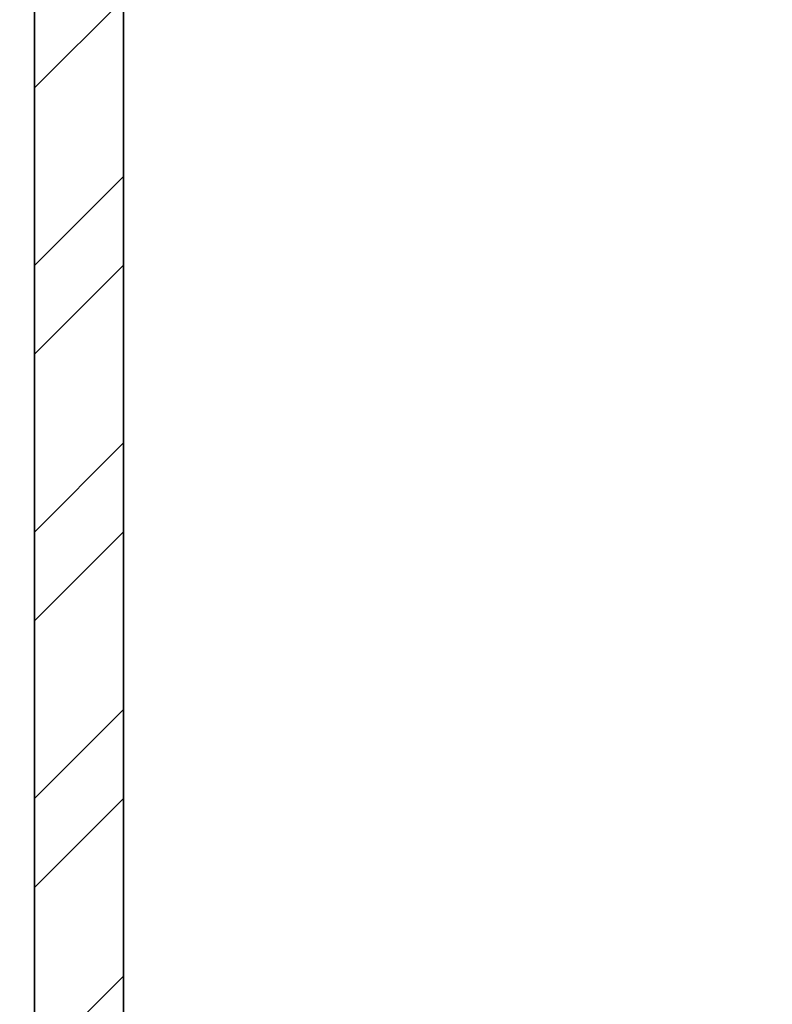
# Model space of a CAD drawing. Units: inches. Extents: x 1885 to 2748, y 783 to 2421.
# Tile 107 of 117: x 2486 to 2524, y 1977 to 2027. Entities that reach past the tile are written whole.
import ezdxf

# ---------------------------------------------------------------- set-up
doc = ezdxf.new("R2010")
doc.units = ezdxf.units.IN
doc.layers.add('A-WALL', color=7, linetype='Continuous', lineweight=35)
doc.layers.add('A-WALL-PATT', color=85, linetype='Continuous', lineweight=13, true_color=0x58ba48)

msp = doc.modelspace()

# ---------------------------------------------------------------- hatches: boundary and pattern name
at = {"layer": 'A-WALL-PATT'}
h = msp.add_hatch(dxfattribs=at)
h.set_pattern_fill('ANSI32', color=256)
h.paths.add_polyline_path([(2007.772, 2318.006), (1980.774, 2318.006), (1980.774, 2281.215), (1985.274, 2281.215), (1985.274, 2313.506), (2007.772, 2313.506), (2007.772, 2315.756)])
h.paths.add_polyline_path([(2094.324, 2318.006), (2067.772, 2318.006), (2067.772, 2313.506), (2094.324, 2313.506), (2094.324, 2315.756)])
h.paths.add_polyline_path([(2131.367, 2315.756), (2131.367, 2318.006), (2131.189, 2318.006), (2112.609, 2318.006), (2112.609, 2313.506), (2117.274, 2313.506), (2117.274, 2255.201), (2121.774, 2255.201), (2121.774, 2313.506), (2131.367, 2313.506)])
h.paths.add_polyline_path([(2190.512, 2318.006), (2155.367, 2318.006), (2155.367, 2313.506), (2169.774, 2313.506), (2169.774, 2229.506), (2121.774, 2229.506), (2121.774, 2233.451), (2119.524, 2233.451), (2117.274, 2233.451), (2117.274, 2201.101), (2121.774, 2201.101), (2121.774, 2225.006), (2169.774, 2225.006), (2169.774, 2165.006), (2306.274, 2165.006), (2306.274, 2066.006), (2310.774, 2066.006), (2344.274, 2066.006), (2486.274, 2066.006), (2486.274, 1886.006), (2483.02, 1886.006), (2483.02, 1881.506), (2486.274, 1881.506), (2486.274, 1880.678), (2490.774, 1880.678), (2490.774, 2070.506), (2344.274, 2070.506), (2310.774, 2070.506), (2310.774, 2165.006), (2310.774, 2173.636), (2308.524, 2173.636), (2306.274, 2173.636), (2306.274, 2169.506), (2174.274, 2169.506), (2174.274, 2313.506), (2190.512, 2313.506), (2190.512, 2315.756)])
h.paths.add_polyline_path([(1985.274, 2221.215), (1980.774, 2221.215), (1980.774, 2165.006), (1992.774, 2165.006), (1992.774, 2141.927), (1997.274, 2141.927), (1997.274, 2165.006), (2117.274, 2165.006), (2117.274, 2163.126), (2121.774, 2163.126), (2121.774, 2172.734), (2119.524, 2172.734), (2117.274, 2172.734), (2117.274, 2169.506), (1985.274, 2169.506)])
h.paths.add_polyline_path([(1997.274, 2105.927), (1992.774, 2105.927), (1992.774, 2070.506), (2016.774, 2070.506), (2016.774, 2059.123), (2019.024, 2059.123), (2021.274, 2059.123), (2021.274, 2070.506), (2117.274, 2070.506), (2117.274, 2022.506), (2114.423, 2022.506), (2114.423, 2018.006), (2123.627, 2018.006), (2123.627, 2020.256), (2123.627, 2022.506), (2121.774, 2022.506), (2121.774, 2142.587), (2119.524, 2142.587), (2117.274, 2142.587), (2117.274, 2075.006), (1997.274, 2075.006)])
h.paths.add_polyline_path([(2092.029, 2020.256), (2092.029, 2022.506), (2021.274, 2022.506), (2021.274, 2035.123), (2016.774, 2035.123), (2016.774, 2018.006), (2016.774, 1978.784), (2021.274, 1978.784), (2021.274, 2018.006), (2092.029, 2018.006)])
h.paths.add_polyline_path([(2260.938, 2022.506), (2153.105, 2022.506), (2153.105, 2020.256), (2153.105, 2018.006), (2155.274, 2018.006), (2155.274, 1886.006), (2107.629, 1886.006), (2107.629, 1881.506), (2182.911, 1881.506), (2182.911, 1883.756), (2182.911, 1886.006), (2159.774, 1886.006), (2159.774, 2018.006), (2260.938, 2018.006), (2260.938, 2020.256)])
h.paths.add_polyline_path([(2047.629, 1883.756), (2047.629, 1886.006), (2021.274, 1886.006), (2021.274, 1918.784), (2019.024, 1918.784), (2016.774, 1918.784), (2016.774, 1881.506), (2047.629, 1881.506)])
h.paths.add_polyline_path([(2306.361, 1883.756), (2306.361, 1886.006), (2296.274, 1886.006), (2296.274, 1982.006), (2316.535, 1982.006), (2316.535, 1984.256), (2316.535, 1986.506), (2296.274, 1986.506), (2296.274, 2022.506), (2289.276, 2022.506), (2289.276, 2018.006), (2291.774, 2018.006), (2291.774, 1886.006), (2242.911, 1886.006), (2242.911, 1881.506), (2306.361, 1881.506)], flags=17)
h.paths.add_polyline_path([(1985.274, 1843.006), (2021.6, 1843.006), (2021.534, 1845.441), (2021.477, 1847.506), (1980.774, 1847.506), (1980.774, 1809.446), (1985.274, 1809.446)])
h.paths.add_polyline_path([(2131.482, 1845.256), (2131.482, 1847.506), (2081.534, 1847.506), (2081.534, 1843.006), (2117.274, 1843.006), (2117.274, 1784.147), (2119.524, 1784.147), (2121.774, 1784.147), (2121.774, 1843.006), (2131.482, 1843.006)])
h.paths.add_polyline_path([(2203.886, 1847.506), (2155.482, 1847.506), (2155.482, 1843.006), (2169.774, 1843.006), (2169.774, 1759.006), (2121.774, 1759.006), (2121.774, 1761.457), (2117.274, 1761.457), (2117.274, 1730.429), (2121.774, 1730.429), (2121.774, 1754.506), (2177.421, 1754.506), (2177.421, 1756.756), (2177.421, 1759.006), (2174.274, 1759.006), (2174.274, 1843.006), (2203.886, 1843.006)])
h.paths.add_polyline_path([(2335.554, 1845.256), (2335.554, 1847.506), (2239.886, 1847.506), (2239.886, 1843.006), (2306.274, 1843.006), (2306.274, 1759.006), (2199.486, 1759.006), (2199.486, 1754.506), (2310.774, 1754.506), (2310.774, 1843.006), (2335.554, 1843.006)])
h.paths.add_polyline_path([(2348.774, 2022.506), (2344.274, 2022.506), (2344.274, 1986.506), (2341.681, 1986.506), (2341.681, 1982.006), (2344.274, 1982.006), (2344.274, 1886.006), (2330.361, 1886.006), (2330.361, 1881.506), (2361.627, 1881.506), (2361.627, 1883.756), (2361.627, 1886.006), (2348.774, 1886.006)], flags=17)
h.paths.add_polyline_path([(2283.251, 2315.756), (2283.251, 2318.006), (2238.512, 2318.006), (2238.512, 2313.506), (2283.251, 2313.506)], flags=17)
h.paths.add_polyline_path([(2363.274, 2348.006), (2388.677, 2348.006), (2388.677, 2350.256), (2388.677, 2352.506), (2358.774, 2352.506), (2358.774, 2348.006), (2358.774, 2318.006), (2344.481, 2318.006), (2344.481, 2313.506), (2358.774, 2313.506), (2358.774, 2229.506), (2310.774, 2229.506), (2310.774, 2231.952), (2306.274, 2231.952), (2306.274, 2205.611), (2310.774, 2205.611), (2310.774, 2225.006), (2358.774, 2225.006), (2358.774, 2211.506), (2452.329, 2211.506), (2452.329, 2213.756), (2452.329, 2216.006), (2363.274, 2216.006), (2363.274, 2318.006)])
h.paths.add_polyline_path([(2310.774, 2313.506), (2320.481, 2313.506), (2320.481, 2315.756), (2320.481, 2318.006), (2302.728, 2318.006), (2302.728, 2313.506), (2306.274, 2313.506), (2306.274, 2251.076), (2310.774, 2251.076)], flags=17)
h.paths.add_polyline_path([(2490.774, 2352.506), (2486.274, 2352.506), (2448.677, 2352.506), (2448.677, 2348.006), (2486.274, 2348.006), (2486.274, 2318.006), (2486.274, 2216.006), (2481.78, 2216.006), (2481.78, 2211.506), (2486.274, 2211.506), (2486.274, 2165.006), (2493.289, 2165.006), (2493.289, 2167.256), (2493.289, 2169.506), (2490.774, 2169.506), (2490.774, 2313.506), (2494.429, 2313.506), (2494.429, 2318.006), (2490.774, 2318.006)])
h.paths.add_polyline_path([(2534.653, 2318.006), (2515.691, 2318.006), (2515.691, 2313.506), (2534.653, 2313.506), (2534.653, 2315.756)])
h.paths.add_polyline_path([(2618.274, 2318.006), (2594.653, 2318.006), (2594.653, 2313.506), (2613.774, 2313.506), (2613.774, 2281.706), (2618.274, 2281.706)])
h.paths.add_polyline_path([(2618.274, 2221.706), (2613.774, 2221.706), (2613.774, 2169.506), (2554.019, 2169.506), (2554.019, 2165.006), (2613.774, 2165.006), (2613.774, 2152.878), (2618.274, 2152.878)])
h.paths.add_polyline_path([(2618.274, 2128.878), (2616.024, 2128.878), (2613.774, 2128.878), (2613.774, 2117.006), (2529.774, 2117.006), (2529.774, 2165.006), (2532.848, 2165.006), (2532.848, 2169.506), (2522.867, 2169.506), (2522.867, 2165.006), (2525.274, 2165.006), (2525.274, 2117.006), (2525.274, 2112.506), (2525.274, 2108.576), (2529.774, 2108.576), (2529.774, 2112.506), (2613.774, 2112.506), (2613.774, 2080.19), (2618.274, 2080.19)])
h.paths.add_polyline_path([(2618.274, 2044.19), (2616.024, 2044.19), (2613.774, 2044.19), (2613.774, 2015.506), (2529.774, 2015.506), (2529.774, 2088.582), (2527.524, 2088.582), (2525.274, 2088.582), (2525.274, 2011.006), (2613.774, 2011.006), (2613.774, 1956.755), (2618.274, 1956.755)])
h.paths.add_polyline_path([(2618.274, 1881.506), (2618.274, 1896.755), (2613.774, 1896.755), (2613.774, 1881.506), (2613.774, 1847.506), (2592.715, 1847.506), (2592.715, 1843.006), (2613.774, 1843.006), (2613.774, 1765.006), (2613.774, 1760.506), (2609.621, 1760.506), (2609.621, 1756.006), (2613.774, 1756.006), (2613.774, 1660.006), (2608.544, 1660.006), (2608.544, 1655.506), (2613.774, 1655.506), (2613.774, 1508.158), (2618.274, 1508.158)])
h.paths.add_polyline_path([(2565.774, 1843.006), (2568.997, 1843.006), (2568.997, 1847.506), (2490.774, 1847.506), (2490.774, 1849.7), (2488.524, 1849.7), (2486.274, 1849.7), (2486.274, 1847.506), (2477.274, 1847.506), (2477.274, 1838.506), (2477.274, 1821.493), (2486.274, 1821.493), (2486.274, 1838.506), (2561.274, 1838.506), (2561.274, 1765.006), (2486.274, 1765.006), (2486.274, 1786.157), (2477.274, 1786.157), (2477.274, 1765.006), (2477.274, 1756.006), (2486.274, 1756.006), (2565.774, 1756.006), (2585.621, 1756.006), (2585.621, 1758.256), (2585.621, 1760.506), (2565.774, 1760.506), (2565.774, 1765.006)])
h.paths.add_polyline_path([(2486.274, 1651.006), (2561.274, 1651.006), (2561.274, 1567.006), (2486.274, 1567.006), (2486.274, 1591.321), (2477.274, 1591.321), (2477.274, 1567.006), (2477.274, 1558.006), (2477.274, 1555.439), (2481.774, 1555.439), (2481.774, 1558.006), (2568.653, 1558.006), (2568.653, 1560.256), (2568.653, 1562.506), (2565.774, 1562.506), (2565.774, 1655.506), (2584.544, 1655.506), (2584.544, 1657.756), (2584.544, 1660.006), (2565.774, 1660.006), (2486.274, 1660.006), (2477.274, 1660.006), (2477.274, 1651.006), (2477.274, 1632.989), (2486.274, 1632.989)])
h.paths.add_polyline_path([(2449.967, 1883.756), (2449.967, 1886.006), (2421.627, 1886.006), (2421.627, 1881.506), (2449.967, 1881.506)], flags=17)
h.paths.add_polyline_path([(2447.274, 1847.506), (2395.554, 1847.506), (2395.554, 1843.006), (2442.774, 1843.006), (2442.774, 1809.27), (2447.274, 1809.27)])
h.paths.add_polyline_path([(1985.274, 1749.446), (1980.774, 1749.446), (1980.774, 1694.504), (1985.274, 1694.504), (1985.274, 1694.506), (1986.897, 1694.506), (1986.897, 1697.78), (1986.897, 1699.006), (1985.274, 1699.006)])
h.paths.add_polyline_path([(2152.774, 1699.006), (2121.774, 1699.006), (2121.774, 1703.668), (2119.524, 1703.668), (2117.274, 1703.668), (2117.274, 1699.006), (2009.219, 1699.006), (2009.219, 1694.506), (2148.274, 1694.506), (2148.274, 1692.631), (2152.774, 1692.631)])
h.paths.add_polyline_path([(2016.274, 1694.506), (2011.774, 1694.506), (2011.774, 1558.006), (2040.806, 1558.006), (2040.806, 1560.256), (2040.806, 1562.506), (2016.274, 1562.506)])
h.paths.add_polyline_path([(2152.774, 1663.017), (2150.524, 1663.017), (2148.274, 1663.017), (2148.274, 1562.506), (2100.806, 1562.506), (2100.806, 1558.006), (2165.119, 1558.006), (2165.119, 1560.256), (2165.119, 1562.506), (2152.774, 1562.506), (2152.774, 1610.506), (2224.774, 1610.506), (2224.774, 1607.99), (2229.274, 1607.99), (2229.274, 1615.006), (2152.774, 1615.006)])
h.paths.add_polyline_path([(2238.613, 1560.256), (2238.613, 1562.506), (2229.274, 1562.506), (2229.274, 1588.756), (2227.024, 1588.763), (2224.774, 1588.771), (2224.774, 1562.506), (2189.119, 1562.506), (2189.119, 1558.006), (2238.613, 1558.006)])
h.paths.add_polyline_path([(2336.024, 1560.256), (2336.024, 1562.506), (2310.774, 1562.506), (2310.774, 1656.347), (2308.524, 1656.347), (2306.274, 1656.347), (2306.274, 1562.506), (2286.613, 1562.506), (2286.613, 1558.006), (2336.024, 1558.006)])
h.paths.add_polyline_path([(2447.274, 1690.968), (2445.024, 1690.968), (2442.774, 1690.968), (2442.774, 1687.006), (2306.274, 1687.006), (2306.274, 1680.75), (2310.774, 1680.75), (2310.774, 1682.506), (2442.774, 1682.506), (2442.774, 1562.506), (2396.024, 1562.506), (2396.024, 1558.006), (2447.274, 1558.006)])
h.paths.add_polyline_path([(2447.274, 1749.27), (2445.024, 1749.27), (2442.774, 1749.27), (2442.774, 1717.232), (2447.274, 1717.232)])
h.paths.add_polyline_path([(2044.674, 1521.756), (2044.674, 1524.006), (2007.274, 1524.006), (2007.274, 1503.49), (2009.524, 1503.49), (2011.774, 1503.49), (2011.774, 1519.506), (2044.674, 1519.506)])
h.paths.add_polyline_path([(2177.969, 1521.756), (2177.969, 1524.006), (2104.674, 1524.006), (2104.674, 1519.506), (2145.774, 1519.506), (2145.774, 1387.506), (2143.37, 1387.506), (2143.37, 1383.006), (2251.585, 1383.006), (2251.585, 1385.256), (2251.585, 1387.506), (2150.274, 1387.506), (2150.274, 1519.506), (2177.969, 1519.506)])
h.paths.add_polyline_path([(2298.704, 1524.006), (2237.969, 1524.006), (2237.969, 1519.506), (2282.274, 1519.506), (2282.274, 1387.506), (2279.683, 1387.506), (2279.683, 1383.006), (2286.774, 1383.006), (2286.774, 1419.006), (2312.451, 1419.006), (2312.451, 1421.256), (2312.451, 1423.506), (2286.774, 1423.506), (2286.774, 1519.506), (2298.704, 1519.506), (2298.704, 1521.722)], flags=17)
h.paths.add_polyline_path([(2361.897, 1521.756), (2361.897, 1524.006), (2322.704, 1524.006), (2322.704, 1519.506), (2334.774, 1519.506), (2334.774, 1423.506), (2331.93, 1423.506), (2331.93, 1419.006), (2334.774, 1419.006), (2334.774, 1387.506), (2334.774, 1383.228), (2339.274, 1383.228), (2339.274, 1387.506), (2339.274, 1519.506), (2361.897, 1519.506)], flags=17)
h.paths.add_polyline_path([(2447.274, 1521.756), (2447.274, 1524.006), (2421.897, 1524.006), (2421.897, 1519.506), (2447.274, 1519.506)], flags=17)
h.paths.add_polyline_path([(2481.774, 1529.6), (2479.524, 1529.6), (2477.274, 1529.6), (2477.274, 1524.006), (2474.489, 1524.006), (2474.489, 1519.506), (2477.274, 1519.506), (2477.274, 1334.506), (2296.774, 1334.506), (2296.774, 1240.506), (2160.274, 1240.506), (2160.274, 1180.506), (2112.274, 1180.506), (2112.274, 1207.692), (2110.024, 1207.692), (2107.774, 1207.692), (2107.774, 1171.609), (2112.274, 1171.609), (2112.274, 1176.006), (2160.274, 1176.006), (2160.274, 1092.006), (2144.221, 1092.006), (2144.221, 1087.506), (2189.497, 1087.506), (2189.497, 1089.756), (2189.497, 1092.006), (2164.774, 1092.006), (2164.774, 1236.006), (2296.774, 1236.006), (2296.774, 1231.912), (2301.274, 1231.912), (2301.274, 1330.006), (2481.774, 1330.006), (2481.774, 1387.506)])
h.paths.add_polyline_path([(2618.274, 1448.158), (2613.774, 1448.158), (2613.774, 1382.506), (2529.774, 1382.506), (2525.274, 1382.506), (2525.274, 1307.062), (2529.774, 1307.062), (2529.774, 1378.006), (2613.774, 1378.006), (2613.774, 1354.988), (2618.274, 1354.988)])
h.paths.add_polyline_path([(2618.274, 1318.988), (2613.774, 1318.988), (2613.774, 1281.006), (2529.774, 1281.006), (2529.774, 1283.786), (2527.524, 1283.786), (2525.274, 1283.786), (2525.274, 1228.506), (2516.794, 1228.506), (2516.794, 1224.006), (2533.484, 1224.006), (2533.484, 1226.256), (2533.484, 1228.506), (2529.774, 1228.506), (2529.774, 1276.506), (2613.774, 1276.506), (2613.774, 1266.02), (2618.274, 1266.02)])
h.paths.add_polyline_path([(2618.274, 1134.964), (2613.774, 1134.964), (2613.774, 1092.006), (2594.545, 1092.006), (2594.545, 1087.506), (2618.274, 1087.506)])
h.paths.add_polyline_path([(2534.545, 1092.006), (2509.765, 1092.006), (2509.765, 1087.506), (2534.545, 1087.506), (2534.545, 1089.756)])
h.paths.add_polyline_path([(2481.274, 1224.006), (2484.117, 1224.006), (2484.117, 1226.256), (2484.117, 1228.506), (2476.774, 1228.506), (2476.774, 1198.506), (2471.61, 1198.506), (2471.61, 1194.006), (2476.774, 1194.006), (2476.774, 1062.006), (2436.894, 1062.006), (2436.894, 1057.506), (2476.774, 1057.506), (2481.274, 1057.506), (2481.274, 1062.006), (2481.274, 1087.506), (2485.354, 1087.506), (2485.354, 1089.756), (2485.354, 1092.006), (2481.274, 1092.006), (2481.274, 1117.506)])
h.paths.add_polyline_path([(2439.898, 1198.506), (2349.274, 1198.506), (2349.274, 1194.006), (2349.274, 1180.506), (2301.274, 1180.506), (2301.274, 1201.896), (2299.024, 1201.896), (2296.774, 1201.896), (2296.774, 1172.335), (2299.024, 1172.335), (2301.274, 1172.335), (2301.274, 1176.006), (2349.274, 1176.006), (2349.274, 1092.006), (2334.452, 1092.006), (2334.452, 1087.506), (2349.274, 1087.506), (2349.274, 1057.506), (2353.774, 1057.506), (2376.894, 1057.506), (2376.894, 1059.756), (2376.894, 1062.006), (2353.774, 1062.006), (2353.774, 1087.506), (2353.774, 1180.506), (2353.774, 1194.006), (2439.898, 1194.006), (2439.898, 1196.256)])
h.paths.add_polyline_path([(2270.596, 1089.756), (2270.596, 1092.006), (2249.497, 1092.006), (2249.497, 1087.506), (2270.596, 1087.506)], flags=17)
h.paths.add_polyline_path([(2310.452, 1092.006), (2301.274, 1092.006), (2301.274, 1153.292), (2296.774, 1153.292), (2296.774, 1092.006), (2293.786, 1092.006), (2293.786, 1087.506), (2310.452, 1087.506), (2310.452, 1089.756)], flags=17)
h.paths.add_polyline_path([(2112.274, 1150.328), (2110.024, 1150.328), (2107.774, 1150.328), (2107.774, 1092.006), (2104.465, 1092.006), (2104.465, 1087.506), (2120.221, 1087.506), (2120.221, 1089.756), (2120.221, 1092.006), (2112.274, 1092.006)])
h.paths.add_polyline_path([(2082.172, 1092.006), (2058.144, 1092.006), (2058.144, 1087.506), (2082.172, 1087.506), (2082.172, 1089.756)])
h.paths.add_polyline_path([(1975.774, 1145.638), (1971.274, 1145.638), (1971.274, 1087.506), (1980.774, 1087.506), (1998.144, 1087.506), (1998.144, 1089.756), (1998.144, 1092.006), (1985.274, 1092.006), (1975.774, 1092.006)])
h.paths.add_polyline_path([(2112.274, 1244.385), (2110.024, 1244.385), (2107.774, 1244.385), (2107.774, 1240.506), (1992.274, 1240.506), (1992.274, 1271.008), (1987.774, 1271.008), (1987.774, 1240.506), (1980.774, 1240.506), (1975.774, 1240.506), (1971.274, 1240.506), (1971.274, 1205.638), (1975.774, 1205.638), (1975.774, 1236.006), (2107.774, 1236.006), (2107.774, 1233.444), (2112.274, 1233.444), (2112.274, 1236.006)])
h.paths.add_polyline_path([(2112.274, 1383.006), (2114.783, 1383.006), (2114.783, 1385.256), (2114.783, 1387.506), (2102.476, 1387.506), (2102.476, 1383.006), (2107.774, 1383.006), (2107.774, 1335.006), (2011.774, 1335.006), (2011.774, 1349.939), (2007.274, 1349.939), (2007.274, 1335.006), (1987.774, 1335.006), (1987.774, 1330.506), (1987.774, 1307.008), (1992.274, 1307.008), (1992.274, 1330.506), (2007.274, 1330.506), (2107.774, 1330.506), (2107.774, 1264.711), (2112.274, 1264.711)])
h.paths.add_polyline_path([(2077.857, 1387.506), (2011.774, 1387.506), (2011.774, 1390.036), (2009.524, 1390.036), (2007.274, 1390.036), (2007.274, 1373.939), (2011.774, 1373.939), (2011.774, 1383.006), (2077.857, 1383.006)])
h.paths.add_polyline_path([(2011.774, 1443.49), (2007.274, 1443.49), (2007.274, 1410.248), (2011.774, 1410.248)])

# ---------------------------------------------------------------- linework, layer by layer
at = {"layer": 'A-WALL'}
for p, q in [((2490.774, 2070.506), (2490.774, 1879.236)), ((2486.274, 2066.006), (2486.274, 1886.006))]:
    msp.add_line(p, q, dxfattribs=at)

doc.saveas('drawing.dxf')
